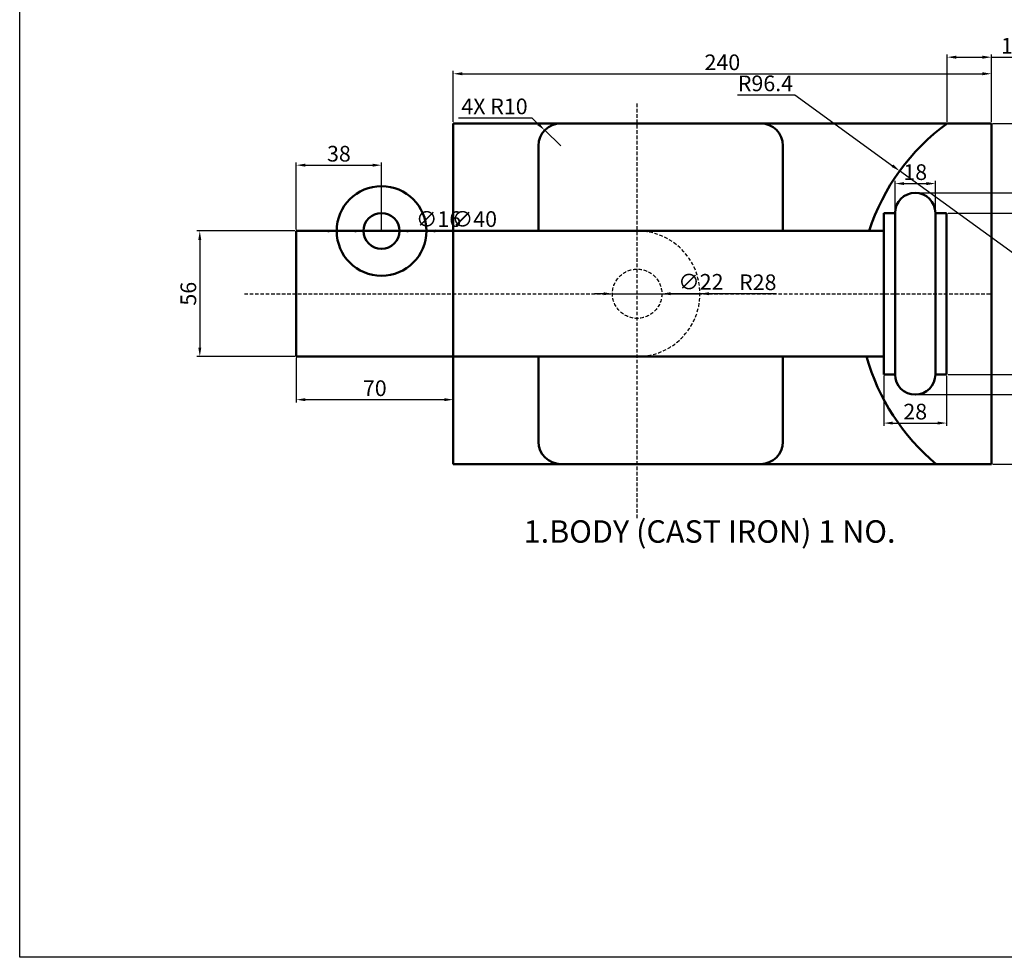
# Model space of a CAD drawing. Units: millimetres. Extents: x -66 to 1195, y -396 to 398.
# Tile 1 of 8: x -66 to 373, y -396 to 23. Entities that reach past the tile are written whole.
import ezdxf

# ---------------------------------------------------------------- set-up
doc = ezdxf.new("R2010")
doc.units = ezdxf.units.MM
doc.header["$LTSCALE"] = 0.5
doc.linetypes.add('HIDDEN', pattern=[9.525, 6.35, -3.175])
for name, color, linetype, lineweight in [('M-DIMS', 2, 'Continuous', 25), ('M-HIDN', 3, 'HIDDEN', 25), ('M-OUTL', 7, 'Continuous', 50), ('M-TEXT', 7, 'Continuous', 25), ('M-TTLB', 7, 'Continuous', 25)]:
    doc.layers.add(name, color=color, linetype=linetype, lineweight=lineweight)
doc.styles.get("Standard").update_dxf_attribs({"font": 'arial.ttf'})
doc.dimstyles.new('ISO-25', dxfattribs={"dimtxt": 7, "dimasz": 4, "dimexe": 1.25, "dimexo": 0.625, "dimtad": 1, "dimtoh": 1, "dimtxsty": 'Standard', "dimcen": 2.5, "dimadec": 0, "dimazin": 0, "dimtfac": 1, "dimtmove": 0, "dimatfit": 3, "dimfxl": 1, "dimarcsym": 0})

# ---------------------------------------------------------------- blocks, each defined once
blk = doc.blocks.new('*D22')
at = {"layer": 'Defpoints', "color": 0, "ltscale": 0.5, "transparency": 16777216}
for p in [(341.94, -50.52), (323.94, -63.65), (341.94, -63.65)]:
    blk.add_point(p, dxfattribs=at)
at = {"layer": 'M-DIMS', "color": 0, "lineweight": -2, "ltscale": 0.5, "transparency": 16777216}
for p, q in [((323.94, -63.03), (323.94, -49.27)), ((327.94, -50.52), (337.94, -50.52)), ((341.94, -63.03), (341.94, -49.27))]:
    blk.add_line(p, q, dxfattribs=at)
at = {"layer": 'M-DIMS', "color": 0, "ltscale": 0.5, "transparency": 16777216}
for points in [[(327.94, -49.85), (327.94, -51.18), (323.94, -50.52)], [(337.94, -49.85), (337.94, -51.18), (341.94, -50.52)]]:
    blk.add_solid(points, dxfattribs=at)
at = {"layer": 'M-DIMS', "color": 0, "ltscale": 0.5, "transparency": 16777216, "insert": (332.94, -46.32), "char_height": 7, "attachment_point": 5}
blk.add_mtext('18', dxfattribs=at)
blk = doc.blocks.new('*D23')
at = {"layer": 'Defpoints', "color": 0, "ltscale": 0.5, "transparency": 16777216}
for p in [(346.94, -63.65), (346.94, -135.65), (387.75, -135.65)]:
    blk.add_point(p, dxfattribs=at)
at = {"layer": 'M-DIMS', "color": 0, "lineweight": -2, "ltscale": 0.5, "transparency": 16777216}
for p, q in [((347.56, -63.65), (389, -63.65)), ((387.75, -67.65), (387.75, -131.65)), ((347.56, -135.65), (389, -135.65))]:
    blk.add_line(p, q, dxfattribs=at)
at = {"layer": 'M-DIMS', "color": 0, "ltscale": 0.5, "transparency": 16777216}
for points in [[(387.08, -67.65), (388.41, -67.65), (387.75, -63.65)], [(387.08, -131.65), (388.41, -131.65), (387.75, -135.65)]]:
    blk.add_solid(points, dxfattribs=at)
at = {"layer": 'M-DIMS', "color": 0, "ltscale": 0.5, "transparency": 16777216, "insert": (383.35, -99.65), "char_height": 7, "attachment_point": 5, "rotation": 90}
blk.add_mtext('%%C72', dxfattribs=at)
blk = doc.blocks.new('*D24')
at = {"layer": 'Defpoints', "color": 0, "ltscale": 0.5, "transparency": 16777216}
for p in [(332.94, -54.65), (332.94, -144.65), (403.33, -144.65)]:
    blk.add_point(p, dxfattribs=at)
at = {"layer": 'M-DIMS', "color": 0, "lineweight": -2, "ltscale": 0.5, "transparency": 16777216}
for p, q in [((333.56, -54.65), (404.58, -54.65)), ((403.33, -58.65), (403.33, -140.65)), ((333.56, -144.65), (404.58, -144.65))]:
    blk.add_line(p, q, dxfattribs=at)
at = {"layer": 'M-DIMS', "color": 0, "ltscale": 0.5, "transparency": 16777216}
for points in [[(402.67, -58.65), (404, -58.65), (403.33, -54.65)], [(402.67, -140.65), (404, -140.65), (403.33, -144.65)]]:
    blk.add_solid(points, dxfattribs=at)
at = {"layer": 'M-DIMS', "color": 0, "ltscale": 0.5, "transparency": 16777216, "insert": (399.13, -99.65), "char_height": 7, "attachment_point": 5, "rotation": 90}
blk.add_mtext('90', dxfattribs=at)
blk = doc.blocks.new('*D25')
at = {"layer": 'Defpoints', "color": 0, "ltscale": 0.5, "transparency": 16777216}
for p in [(366.94, -23.65), (366.94, -175.65), (420.24, -175.65)]:
    blk.add_point(p, dxfattribs=at)
at = {"layer": 'M-DIMS', "color": 0, "lineweight": -2, "ltscale": 0.5, "transparency": 16777216}
for p, q in [((367.56, -23.65), (421.49, -23.65)), ((420.24, -27.65), (420.24, -171.65)), ((367.56, -175.65), (421.49, -175.65))]:
    blk.add_line(p, q, dxfattribs=at)
at = {"layer": 'M-DIMS', "color": 0, "ltscale": 0.5, "transparency": 16777216}
for points in [[(419.57, -27.65), (420.9, -27.65), (420.24, -23.65)], [(419.57, -171.65), (420.9, -171.65), (420.24, -175.65)]]:
    blk.add_solid(points, dxfattribs=at)
at = {"layer": 'M-DIMS', "color": 0, "ltscale": 0.5, "transparency": 16777216, "insert": (416.04, -99.65), "char_height": 7, "attachment_point": 5, "rotation": 90}
blk.add_mtext('152', dxfattribs=at)
blk = doc.blocks.new('*D26')
at = {"layer": 'Defpoints', "color": 0, "ltscale": 0.5, "transparency": 16777216}
for p in [(366.94, -1.52), (126.94, -23.65), (366.94, -23.65)]:
    blk.add_point(p, dxfattribs=at)
at = {"layer": 'M-DIMS', "color": 0, "lineweight": -2, "ltscale": 0.5, "transparency": 16777216}
for p, q in [((126.94, -23.03), (126.94, -0.27)), ((130.94, -1.52), (362.94, -1.52)), ((366.94, -23.03), (366.94, -0.27))]:
    blk.add_line(p, q, dxfattribs=at)
at = {"layer": 'M-DIMS', "color": 0, "ltscale": 0.5, "transparency": 16777216}
for points in [[(130.94, -0.85), (130.94, -2.19), (126.94, -1.52)], [(362.94, -0.85), (362.94, -2.19), (366.94, -1.52)]]:
    blk.add_solid(points, dxfattribs=at)
at = {"layer": 'M-DIMS', "color": 0, "ltscale": 0.5, "transparency": 16777216, "insert": (246.94, 2.68), "char_height": 7, "attachment_point": 5}
blk.add_mtext('240', dxfattribs=at)
blk = doc.blocks.new('*D27')
at = {"layer": 'Defpoints', "color": 0, "ltscale": 0.5, "transparency": 16777216}
for p in [(94.94, -42.3), (56.94, -71.65), (94.94, -71.65)]:
    blk.add_point(p, dxfattribs=at)
at = {"layer": 'M-DIMS', "color": 0, "lineweight": -2, "ltscale": 0.5, "transparency": 16777216}
for p, q in [((56.94, -71.03), (56.94, -41.05)), ((60.94, -42.3), (90.94, -42.3)), ((94.94, -71.03), (94.94, -41.05))]:
    blk.add_line(p, q, dxfattribs=at)
at = {"layer": 'M-DIMS', "color": 0, "ltscale": 0.5, "transparency": 16777216}
for points in [[(60.94, -41.64), (60.94, -42.97), (56.94, -42.3)], [(90.94, -41.64), (90.94, -42.97), (94.94, -42.3)]]:
    blk.add_solid(points, dxfattribs=at)
at = {"layer": 'M-DIMS', "color": 0, "ltscale": 0.5, "transparency": 16777216, "insert": (75.94, -38.1), "char_height": 7, "attachment_point": 5}
blk.add_mtext('38', dxfattribs=at)
blk = doc.blocks.new('*D28')
at = {"layer": 'Defpoints', "color": 0, "ltscale": 0.5, "transparency": 16777216}
for p in [(56.94, -127.65), (126.94, -137.46), (126.94, -146.91)]:
    blk.add_point(p, dxfattribs=at)
at = {"layer": 'M-DIMS', "color": 0, "lineweight": -2, "ltscale": 0.5, "transparency": 16777216}
for p, q in [((56.94, -128.28), (56.94, -148.16)), ((126.94, -138.08), (126.94, -148.16)), ((60.94, -146.91), (122.94, -146.91))]:
    blk.add_line(p, q, dxfattribs=at)
at = {"layer": 'M-DIMS', "color": 0, "ltscale": 0.5, "transparency": 16777216}
for points in [[(60.94, -146.25), (60.94, -147.58), (56.94, -146.91)], [(122.94, -146.25), (122.94, -147.58), (126.94, -146.91)]]:
    blk.add_solid(points, dxfattribs=at)
at = {"layer": 'M-DIMS', "color": 0, "ltscale": 0.5, "transparency": 16777216, "insert": (91.94, -142.71), "char_height": 7, "attachment_point": 5}
blk.add_mtext('70', dxfattribs=at)
blk = doc.blocks.new('*D29')
at = {"layer": 'Defpoints', "color": 0, "ltscale": 0.5, "transparency": 16777216}
for p in [(318.94, -135.65), (346.94, -135.65), (346.94, -157.35)]:
    blk.add_point(p, dxfattribs=at)
at = {"layer": 'M-DIMS', "color": 0, "lineweight": -2, "ltscale": 0.5, "transparency": 16777216}
for p, q in [((318.94, -136.28), (318.94, -158.6)), ((346.94, -136.28), (346.94, -158.6)), ((322.94, -157.35), (342.94, -157.35))]:
    blk.add_line(p, q, dxfattribs=at)
at = {"layer": 'M-DIMS', "color": 0, "ltscale": 0.5, "transparency": 16777216}
for points in [[(322.94, -156.69), (322.94, -158.02), (318.94, -157.35)], [(342.94, -156.69), (342.94, -158.02), (346.94, -157.35)]]:
    blk.add_solid(points, dxfattribs=at)
at = {"layer": 'M-DIMS', "color": 0, "ltscale": 0.5, "transparency": 16777216, "insert": (332.94, -153.15), "char_height": 7, "attachment_point": 5}
blk.add_mtext('28', dxfattribs=at)
blk = doc.blocks.new('*D105')
at = {"layer": 'Defpoints', "color": 0, "ltscale": 0.5, "transparency": 16777216}
for p in [(56.94, -71.65), (13.9, -127.65), (56.94, -127.65)]:
    blk.add_point(p, dxfattribs=at)
at = {"layer": 'M-DIMS', "color": 0, "lineweight": -2, "ltscale": 0.5, "transparency": 16777216}
for p, q in [((56.31, -71.65), (12.65, -71.65)), ((13.9, -75.65), (13.9, -123.65)), ((56.31, -127.65), (12.65, -127.65))]:
    blk.add_line(p, q, dxfattribs=at)
at = {"layer": 'M-DIMS', "color": 0, "ltscale": 0.5, "transparency": 16777216}
for points in [[(13.23, -75.65), (14.56, -75.65), (13.9, -71.65)], [(13.23, -123.65), (14.56, -123.65), (13.9, -127.65)]]:
    blk.add_solid(points, dxfattribs=at)
at = {"layer": 'M-DIMS', "color": 0, "ltscale": 0.5, "transparency": 16777216, "insert": (9.7, -99.65), "char_height": 7, "attachment_point": 5, "rotation": 90}
blk.add_mtext('56', dxfattribs=at)
blk = doc.blocks.new('*D106')
at = {"layer": 'Defpoints', "color": 0, "ltscale": 0.5, "transparency": 16777216}
for p in [(366.94, 5.88), (347.21, -23.65), (366.94, -23.65)]:
    blk.add_point(p, dxfattribs=at)
at = {"layer": 'M-DIMS', "color": 0, "lineweight": -2, "ltscale": 0.5, "transparency": 16777216}
for p, q in [((347.21, -23.03), (347.21, 7.13)), ((351.21, 5.88), (362.94, 5.88)), ((366.94, -23.03), (366.94, 7.13)), ((366.94, 5.88), (400.59, 5.88))]:
    blk.add_line(p, q, dxfattribs=at)
at = {"layer": 'M-DIMS', "color": 0, "ltscale": 0.5, "transparency": 16777216}
for points in [[(351.21, 6.55), (351.21, 5.21), (347.21, 5.88)], [(362.94, 6.55), (362.94, 5.21), (366.94, 5.88)]]:
    blk.add_solid(points, dxfattribs=at)
at = {"layer": 'M-DIMS', "color": 0, "ltscale": 0.5, "transparency": 16777216, "insert": (385.76, 10.08), "char_height": 7, "attachment_point": 5}
blk.add_mtext('19.727', dxfattribs=at)
blk = doc.blocks.new('*D119')
at = {"layer": 'Defpoints', "color": 0, "ltscale": 0.5, "transparency": 16777216}
for p in [(74.94, -71.66), (114.94, -71.65)]:
    blk.add_point(p, dxfattribs=at)
at = {"layer": 'M-DIMS', "color": 0, "lineweight": -2, "ltscale": 0.5, "transparency": 16777216}
for p, q in [((70.94, -71.66), (66.94, -71.66)), ((74.94, -71.66), (114.94, -71.65)), ((126.94, -71.65), (118.94, -71.65)), ((145.18, -71.65), (126.94, -71.65))]:
    blk.add_line(p, q, dxfattribs=at)
at = {"layer": 'M-DIMS', "color": 0, "ltscale": 0.5, "transparency": 16777216}
for points in [[(70.94, -70.99), (70.94, -72.32), (74.94, -71.66)], [(118.94, -70.98), (118.94, -72.32), (114.94, -71.65)]]:
    blk.add_solid(points, dxfattribs=at)
at = {"layer": 'M-DIMS', "color": 0, "ltscale": 0.5, "transparency": 16777216, "insert": (136.37, -67.25), "char_height": 7, "attachment_point": 5}
blk.add_mtext('∅40', dxfattribs=at)
blk = doc.blocks.new('*D120')
at = {"layer": 'Defpoints', "color": 0, "ltscale": 0.5, "transparency": 16777216}
for p in [(86.94, -71.66), (102.94, -71.65)]:
    blk.add_point(p, dxfattribs=at)
at = {"layer": 'M-DIMS', "color": 0, "lineweight": -2, "ltscale": 0.5, "transparency": 16777216}
for p, q in [((82.94, -71.66), (78.94, -71.66)), ((86.94, -71.66), (102.94, -71.65)), ((110.94, -71.65), (106.94, -71.65)), ((129.2, -71.65), (110.94, -71.65))]:
    blk.add_line(p, q, dxfattribs=at)
at = {"layer": 'M-DIMS', "color": 0, "ltscale": 0.5, "transparency": 16777216}
for points in [[(82.94, -70.99), (82.94, -72.32), (86.94, -71.66)], [(106.94, -70.98), (106.94, -72.31), (102.94, -71.65)]]:
    blk.add_solid(points, dxfattribs=at)
at = {"layer": 'M-DIMS', "color": 0, "ltscale": 0.5, "transparency": 16777216, "insert": (120.38, -67.25), "char_height": 7, "attachment_point": 5}
blk.add_mtext('∅16', dxfattribs=at)
blk = doc.blocks.new('*D121')
at = {"layer": 'Defpoints', "color": 0, "ltscale": 0.5, "transparency": 16777216}
for p in [(325.99, -44.9), (403.98, -101.56)]:
    blk.add_point(p, dxfattribs=at)
at = {"layer": 'M-DIMS', "color": 0, "lineweight": -2, "ltscale": 0.5, "transparency": 16777216}
for p, q in [((253.72, -10.91), (279.2, -10.91)), ((279.2, -10.91), (322.76, -42.55)), ((403.98, -101.56), (325.99, -44.9))]:
    blk.add_line(p, q, dxfattribs=at)
at = {"layer": 'M-DIMS', "color": 0, "ltscale": 0.5, "transparency": 16777216}
blk.add_solid([(323.15, -42.01), (322.36, -43.09), (325.99, -44.9)], dxfattribs=at)
at = {"layer": 'M-DIMS', "color": 0, "ltscale": 0.5, "transparency": 16777216, "insert": (266.15, -6.71), "char_height": 7, "attachment_point": 5}
blk.add_mtext('R96.4', dxfattribs=at)
blk = doc.blocks.new('*D122')
at = {"layer": 'Defpoints', "color": 0, "ltscale": 0.5, "transparency": 16777216}
for p in [(197.94, -99.66), (219.94, -99.65)]:
    blk.add_point(p, dxfattribs=at)
at = {"layer": 'M-DIMS', "color": 0, "lineweight": -2, "ltscale": 0.5, "transparency": 16777216}
for p, q in [((193.94, -99.66), (189.94, -99.66)), ((197.94, -99.66), (219.94, -99.65)), ((227.94, -99.65), (223.94, -99.65)), ((246.13, -99.65), (227.94, -99.65))]:
    blk.add_line(p, q, dxfattribs=at)
at = {"layer": 'M-DIMS', "color": 0, "ltscale": 0.5, "transparency": 16777216}
for points in [[(193.94, -98.99), (193.94, -100.32), (197.94, -99.66)], [(223.94, -98.98), (223.94, -100.32), (219.94, -99.65)]]:
    blk.add_solid(points, dxfattribs=at)
at = {"layer": 'M-DIMS', "color": 0, "ltscale": 0.5, "transparency": 16777216, "insert": (237.35, -95.25), "char_height": 7, "attachment_point": 5}
blk.add_mtext('∅22', dxfattribs=at)
blk = doc.blocks.new('*D123')
at = {"layer": 'Defpoints', "color": 0, "ltscale": 0.5, "transparency": 16777216}
for p in [(208.94, -99.65), (236.94, -99.65)]:
    blk.add_point(p, dxfattribs=at)
at = {"layer": 'M-DIMS', "color": 0, "lineweight": -2, "ltscale": 0.5, "transparency": 16777216}
for p, q in [((208.94, -99.65), (236.94, -99.65)), ((253.74, -99.65), (240.94, -99.65)), ((271.1, -99.65), (253.74, -99.65))]:
    blk.add_line(p, q, dxfattribs=at)
at = {"layer": 'M-DIMS', "color": 0, "ltscale": 0.5, "transparency": 16777216}
blk.add_solid([(240.94, -98.98), (240.94, -100.32), (236.94, -99.65)], dxfattribs=at)
at = {"layer": 'M-DIMS', "color": 0, "ltscale": 0.5, "transparency": 16777216, "insert": (262.73, -95.45), "char_height": 7, "attachment_point": 5}
blk.add_mtext('R28', dxfattribs=at)
blk = doc.blocks.new('*D124')
at = {"layer": 'Defpoints', "color": 0, "ltscale": 0.5, "transparency": 16777216}
for p in [(167.72, -26.73), (174.94, -33.65)]:
    blk.add_point(p, dxfattribs=at)
at = {"layer": 'M-DIMS', "color": 0, "lineweight": -2, "ltscale": 0.5, "transparency": 16777216}
for p, q in [((129.3, -21.19), (161.95, -21.19)), ((161.95, -21.19), (164.83, -23.96)), ((174.94, -33.65), (167.72, -26.73))]:
    blk.add_line(p, q, dxfattribs=at)
at = {"layer": 'M-DIMS', "color": 0, "ltscale": 0.5, "transparency": 16777216}
blk.add_solid([(165.29, -23.48), (164.37, -24.44), (167.72, -26.73)], dxfattribs=at)
at = {"layer": 'M-DIMS', "color": 0, "ltscale": 0.5, "transparency": 16777216, "insert": (145.31, -16.99), "char_height": 7, "attachment_point": 5}
blk.add_mtext('4X R10', dxfattribs=at)

msp = doc.modelspace()

# ---------------------------------------------------------------- linework, layer by layer
at = {"layer": 'M-HIDN', "ltscale": 0.5}
for p, q in [((208.9367, -199.7441), (208.9367, -14.0209)), ((33.7952, -99.6533), (366.9367, -99.6533))]:
    msp.add_line(p, q, dxfattribs=at)
msp.add_circle((208.9367, -99.6533), 11, dxfattribs=at)
msp.add_arc((208.9367, -99.6533), 28, 270, 90, dxfattribs=at)
at = {"layer": 'M-OUTL', "ltscale": 0.5}
for p, q in [((126.9367, -23.6533), (366.9367, -23.6533)), ((126.9367, -175.6533), (126.9367, -23.6533)), ((366.9367, -23.6533), (366.9367, -175.6533)), ((164.9367, -33.6533), (164.9367, -71.6533)), ((273.9367, -33.6533), (273.9367, -71.6533)), ((318.9367, -63.6533), (318.9367, -135.6533)), ((323.9367, -63.6533), (318.9367, -63.6533)), ((323.9367, -63.6533), (323.9367, -135.6533)), ((346.9367, -63.6533), (341.9367, -63.6533)), ((341.9367, -63.6533), (341.9367, -135.6533)), ((346.9367, -135.6533), (346.9367, -63.6533)), ((56.9367, -127.6533), (56.9367, -71.6533)), ((56.9367, -71.6533), (318.9367, -71.6533)), ((56.9367, -79.6533), (56.9367, -119.6533)), ((56.9367, -127.6533), (318.9367, -127.6533)), ((164.9367, -127.6533), (164.9367, -165.6533)), ((273.9367, -127.6533), (273.9367, -165.6533)), ((318.9367, -135.6533), (323.9367, -135.6533)), ((341.9367, -135.6533), (346.9367, -135.6533)), ((366.9367, -175.6533), (126.9367, -175.6533))]:
    msp.add_line(p, q, dxfattribs=at)
at = {"layer": 'M-OUTL'}
msp.add_line((56.9367, -127.6533), (56.9367, -71.6533), dxfattribs=at)
at = {"layer": 'M-OUTL', "ltscale": 0.5}
for radius in [20, 8]:
    msp.add_circle((94.9367, -71.6533), radius, dxfattribs=at)
for centre, radius, start, end in [((174.9367, -33.6533), 10, 90, 180), ((263.9367, -33.6533), 10, 360, 90), ((403.9811, -101.5567), 96.3948, 126.082432, 161.927611), ((332.9367, -63.6533), 9, 0, 180), ((403.9811, -101.5567), 96.3948, 195.707464, 230.235325), ((332.9367, -135.6533), 9, 180, 0), ((174.9367, -165.6533), 10, 180, 270), ((263.9367, -165.6533), 10, 270, 0)]:
    msp.add_arc(centre, radius, start, end, dxfattribs=at)
at = {"layer": 'M-TTLB', "ltscale": 0.5}
msp.add_lwpolyline([(-66.4176, 397.641), (1195.0519, 397.641), (1195.0519, -395.6964), (-66.4176, -395.6964)], close=True, dxfattribs=at)

# ---------------------------------------------------------------- texts
at = {"layer": 'M-TEXT', "ltscale": 0.5, "insert": (145.5648, -200.7302), "char_height": 10, "attachment_point": 1}
msp.add_mtext_dynamic_manual_height_columns('\\pxqc;1.BODY (CAST IRON) 1 NO.', width=191.333714, gutter_width=12.5, heights=[0], dxfattribs=at)

# ---------------------------------------------------------------- dimensions: what is measured, and where the dimension line sits
at = {"layer": 'M-DIMS', "ltscale": 0.5}
for base, p1, p2, override, picture, middle in [((366.9367, 5.8791), (347.2095, -23.6533), (366.9367, -23.6533), {"dimdec": 3, "dimlfac": 1, "dimrnd": 0, "dimzin": 0, "dimdsep": 46, "dimlunit": 2}, '*D106', (385.7622, 10.0781)), ((366.9367, -1.5208), (126.9367, -23.6533), (366.9367, -23.6533), {"dimclrd": 0, "dimclre": 0, "dimclrt": 0}, '*D26', (246.9367, 2.6782)), ((94.9367, -42.3024), (56.9367, -71.6533), (94.9367, -71.6533), {"dimclrd": 0, "dimclre": 0, "dimclrt": 0}, '*D27', (75.9367, -38.101)), ((341.9367, -50.5182), (323.9367, -63.6533), (341.9367, -63.6533), {"dimclrd": 0, "dimclre": 0, "dimclrt": 0}, '*D22', (332.9367, -46.3192)), ((126.9367, -146.912), (56.9367, -127.6533), (126.9367, -137.4565), {"dimclrd": 0, "dimclre": 0, "dimclrt": 0}, '*D28', (91.9367, -142.713)), ((346.9367, -157.3521), (318.9367, -135.6533), (346.9367, -135.6533), {"dimclrd": 0, "dimclre": 0, "dimclrt": 0}, '*D29', (332.9367, -153.153))]:
    dim = msp.add_linear_dim(base=base, p1=p1, p2=p2, dimstyle='ISO-25', override=override, dxfattribs=at)
    dim.commit()
    dim.dimension.update_dxf_attribs({"geometry": picture, "text_midpoint": middle})
for center, mpoint, override, picture, middle in [((403.9811, -101.5567), (325.9927, -44.9019), {"dimdec": 1, "dimlfac": 1, "dimrnd": 0, "dimzin": 0, "dimdsep": 46, "dimlunit": 2}, '*D121', (266.1479, -10.909)), ((208.9367, -99.6533), (236.9367, -99.65), {"dimdec": 0, "dimlfac": 1, "dimrnd": 0, "dimzin": 0, "dimdsep": 46, "dimlunit": 2}, '*D123', (253.7367, -99.648))]:
    dim = msp.add_radius_dim(center=center, mpoint=mpoint, dimstyle='ISO-25', override=override, dxfattribs=at)
    dim.commit()
    dim.dimension.update_dxf_attribs({"geometry": picture, "text_midpoint": middle, "dimtype": 164})
dim = msp.add_radius_dim(center=(174.9367, -33.6533), mpoint=(167.7197, -26.7312), text='4X <>', dimstyle='ISO-25', override={"dimdec": 0, "dimlfac": 1, "dimrnd": 0, "dimzin": 0, "dimdsep": 46, "dimlunit": 2}, dxfattribs=at)
dim.commit()
dim.dimension.update_dxf_attribs({"geometry": '*D124', "text_midpoint": (145.3086, -16.9945)})
for base, p1, p2, override, picture, middle in [((420.2377, -175.6533), (366.9367, -23.6533), (366.9367, -175.6533), {"dimclrd": 0, "dimclre": 0, "dimclrt": 0}, '*D25', (416.0387, -99.6533)), ((403.3318, -144.6533), (332.9367, -54.6533), (332.9367, -144.6533), {"dimclrd": 0, "dimclre": 0, "dimclrt": 0}, '*D24', (399.1328, -99.6533)), ((13.8952, -127.6533), (56.9367, -71.6533), (56.9367, -127.6533), {"dimdec": 0, "dimlfac": 1, "dimrnd": 0, "dimzin": 0, "dimdsep": 46, "dimlunit": 2}, '*D105', (9.6961, -99.6533))]:
    dim = msp.add_linear_dim(base=base, p1=p1, p2=p2, angle=90, dimstyle='ISO-25', override=override, dxfattribs=at)
    dim.commit()
    dim.dimension.update_dxf_attribs({"geometry": picture, "text_midpoint": middle})
for p1, p2, picture, middle in [((74.9367, -71.6566), (114.9367, -71.65), '*D119', (126.9367, -71.648)), ((197.9367, -99.6566), (219.9367, -99.65), '*D122', (227.9367, -99.6476))]:
    dim = msp.add_diameter_dim_2p(p1=p1, p2=p2, dimstyle='ISO-25', override={"dimdec": 0, "dimlfac": 1, "dimrnd": 0, "dimzin": 0, "dimdsep": 46, "dimlunit": 2}, dxfattribs=at)
    dim.commit()
    dim.dimension.update_dxf_attribs({"geometry": picture, "text_midpoint": middle, "dimtype": 163})
dim = msp.add_diameter_dim_2p(p1=(86.9367, -71.6566), p2=(102.9367, -71.65), dimstyle='ISO-25', override={"dimdec": 0, "dimlfac": 1, "dimrnd": 0, "dimzin": 0, "dimdsep": 46, "dimlunit": 2}, dxfattribs=at)
dim.commit()
dim.dimension.update_dxf_attribs({"geometry": '*D120', "text_midpoint": (110.9367, -71.6467)})
dim = msp.add_linear_dim(base=(387.7471, -135.6533), p1=(346.9367, -63.6533), p2=(346.9367, -135.6533), angle=90, text='%%C<>', dimstyle='ISO-25', override={"dimclrd": 0, "dimclre": 0, "dimclrt": 0}, dxfattribs=at)
dim.commit()
dim.dimension.update_dxf_attribs({"geometry": '*D23', "text_midpoint": (383.3523, -99.6533)})

doc.saveas('drawing.dxf')
